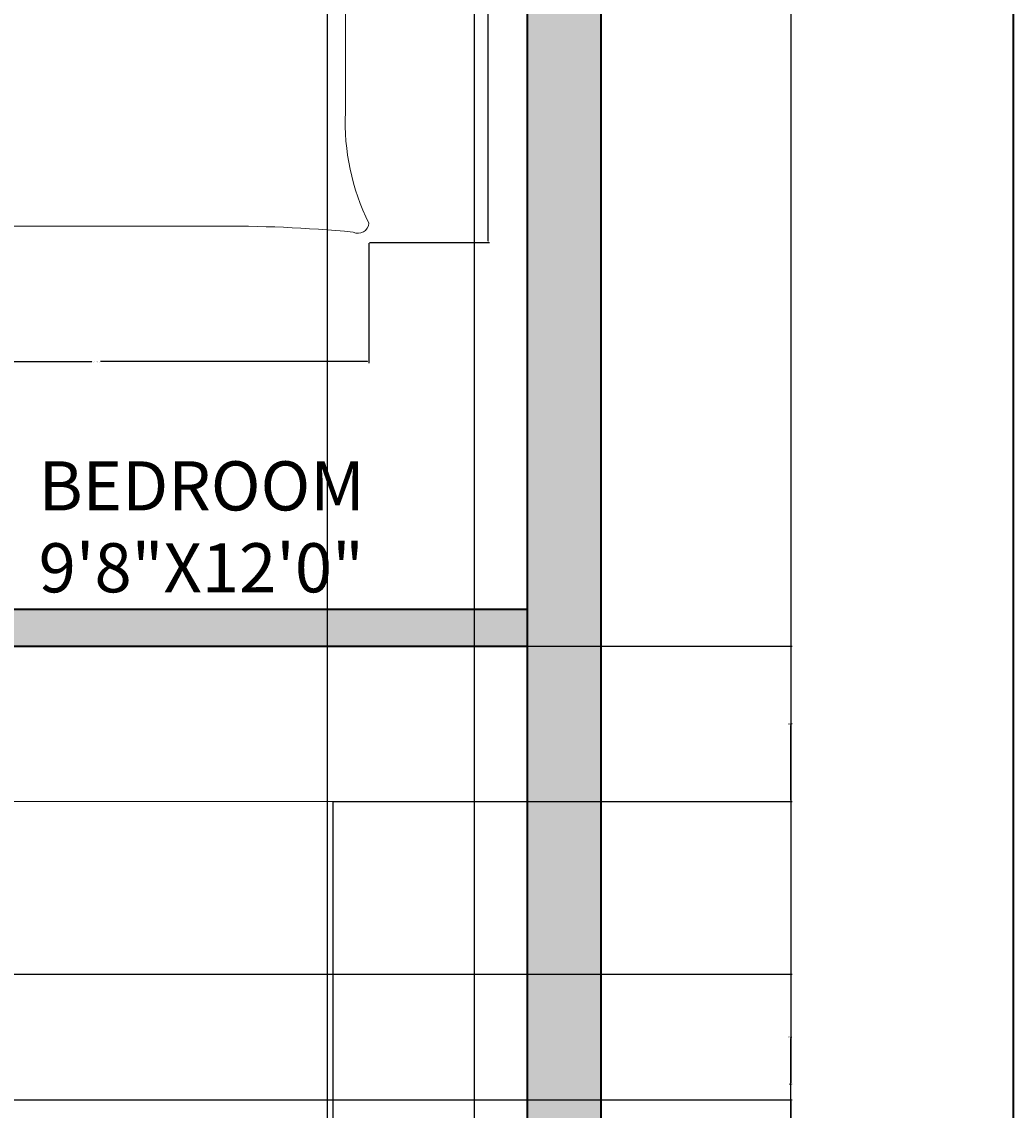
# Model space of a CAD drawing. Units: inches. Extents: x 2606 to 3027, y 1906 to 2463.
# Tile 8 of 10: x 2906 to 3027, y 2196 to 2329. Entities that reach past the tile are written whole.
import ezdxf

# ---------------------------------------------------------------- set-up
doc = ezdxf.new("R2010")
doc.units = ezdxf.units.IN
for name, color, linetype, lineweight in [('A-ANNO-DIMS', 2, 'Continuous', 18), ('A-ANNO-TTLB', 7, 'Continuous', 35), ('A-AREA-IDEN', 7, 'Continuous', 18), ('A-FLOR-CASE', 8, 'Continuous', 18), ('A-FURN', 8, 'Continuous', 13), ('A-WALL', 7, 'Continuous', 35)]:
    doc.layers.add(name, color=color, linetype=linetype, lineweight=lineweight)
doc.layers.add('A-WALL-PATT', color=251, linetype='Continuous', lineweight=13, true_color=0x636466)
doc.styles.get("Standard").update_dxf_attribs({"font": 'arial.ttf'})
doc.dimstyles.get("Standard").update_dxf_attribs({"dimtxt": 0.18, "dimasz": 0.18, "dimexe": 0.18, "dimexo": 0.0625, "dimgap": 0.09, "dimtad": 0, "dimtih": 1, "dimtoh": 1, "dimdec": 4, "dimzin": 0, "dimdsep": 46, "dimtxsty": 'Standard', "dimcen": 0.09, "dimadec": 0, "dimazin": 0, "dimtfac": 1, "dimtdec": 4, "dimtofl": 0, "dimtmove": 0, "dimatfit": 3, "dimfxl": 1, "dimtolj": 1, "dimtzin": 0, "dimarcsym": 0})

# ---------------------------------------------------------------- blocks, each defined once
blk = doc.blocks.new('BED-DOUBLE')
for p, q in [((4.17, 75.16), (4.17, 96.87)), ((4.17, 96.87), (61.46, 96.87)), ((61.46, 96.87), (61.46, 64.97)), ((4.17, 95.03), (61.46, 95.03)), ((29.42, 93.94), (31.15, 94.63)), ((31.15, 94.63), (31.84, 88.22)), ((4.67, 92.87), (9.81, 93.27)), ((9.81, 93.27), (9.93, 93.24)), ((9.93, 93.24), (14.52, 92.9)), ((17.81, 92.38), (20.24, 93.24)), ((20.24, 93.24), (23.7, 94.11)), ((23.7, 94.11), (24.09, 94.11)), ((24.09, 94.11), (29.42, 93.94)), ((33.54, 93.89), (33.25, 87.44)), ((35.31, 93.3), (33.54, 93.89)), ((40.62, 93.81), (35.31, 93.3)), ((41.01, 93.83), (40.62, 93.81)), ((44.52, 93.18), (41.01, 93.83)), ((50.25, 93.19), (43.75, 91.57)), ((47, 92.47), (44.52, 93.18)), ((54.8, 93.82), (50.25, 93.19)), ((60.08, 93.81), (53.6, 93.92)), ((53.6, 93.92), (54.8, 93.82)), ((60.08, 93.81), (59.62, 89.96)), ((4.67, 92.9), (5.36, 89.08)), ((14.52, 92.9), (21.1, 91.68)), ((5.36, 89.08), (4.84, 85.96)), ((6.06, 86.14), (7.27, 89.43)), ((59.12, 86.97), (57.7, 90.18)), ((59.62, 89.96), (60.34, 86.88)), ((31.84, 88.22), (32.54, 84.4)), ((33.25, 87.44), (32.79, 83.59)), ((60.08, 82.69), (59.12, 86.97)), ((60.34, 86.88), (59.72, 85.62)), ((4.84, 85.96), (5.54, 84.75)), ((5.36, 81.8), (6.06, 86.14)), ((32.54, 84.4), (32.54, 82.84)), ((32.54, 82.84), (31.84, 80.59)), ((32.79, 83.59), (32.89, 82.03)), ((59.85, 80.77), (60.08, 82.69)), ((5.71, 79.9), (5.36, 81.8)), ((32.89, 82.03), (33.72, 79.83)), ((5.02, 76.08), (5.71, 79.9)), ((31.84, 80.59), (31.84, 77.38)), ((33.72, 79.83), (33.92, 76.62)), ((60.78, 77), (59.85, 80.77)), ((28.9, 77.38), (25.13, 78.68)), ((7.65, 78.14), (12.48, 77.34)), ((12.48, 77.34), (11.13, 76.95)), ((12.48, 77.34), (20.89, 76.82)), ((20.89, 76.82), (23.24, 77.49)), ((23.24, 77.49), (29.39, 77)), ((31.84, 77.38), (28.9, 77.38)), ((36.87, 76.8), (40.55, 78.34)), ((39.04, 78.14), (43.87, 77.34)), ((43.87, 77.34), (52.28, 76.82)), ((52.28, 76.82), (54.63, 77.49)), ((54.63, 77.49), (60.78, 77)), ((11.13, 76.95), (5.02, 76.08)), ((33.92, 76.62), (36.87, 76.8)), ((36.28, 76.03), (41.3, 68.25)), ((48.73, 72.52), (38.73, 76.03)), ((55.41, 70.1), (48.73, 72.52)), ((58.94, 67.51), (55.41, 70.1)), ((41.3, 68.25), (43.34, 62.87)), ((63.38, 63.61), (58.94, 67.51)), ((43.34, 62.87), (43.71, 60.45)), ((49.1, 62.31), (53.18, 62.87)), ((53.18, 62.87), (57.82, 63.24)), ((57.82, 63.24), (61.54, 62.87)), ((61.54, 62.87), (63.38, 63.61)), ((63.48, 61.52), (63.38, 63.61, 4.64)), ((43.71, 60.45), (46.68, 61.2)), ((46.68, 61.2), (49.1, 62.31)), ((18.06, 1.87), (47.57, 1.87))]:
    blk.add_line(p, q)
for centre, radius, start, end in [((25.61, -121.38), 197.77, 86.0865, 96.7821), ((102.1, 72.78), 99.87, 178.7218, 185.604), ((21.29, -90.53), 154.68, 81.7845, 96.9006), ((-200.58, 59.5), 203.94, 358.4762, 1.0082), ((37.35, 95.1), 35.55, 280.6617, 289.8806), ((52.44, 54.83), 7.46, 78.6608, 113.7384), ((61.53, 104.85), 43.38, 259.8763, 272.5657), ((218.51, 53.34), 155.25, 176.9791, 183.8365), ((43.92, 60.38), 0.221, 160.2464, 271.1377), ((581.23, 36.19), 578.22, 178.22771, 181.71854), ((-5405.34, 15.56), 5469.02, 0.00217, 0.28689), ((-32.25, 19.53), 35.53, 346.0648, 358.9113), ((91.3, 14.55), 27.65, 177.4714, 206.4681), ((-25.97, 12.62), 28.25, 337.9751, 356.652), ((-20.65, 125.3), 127.63, 283.3832, 287.7053), ((1.3, 1.3), 1.31, 146.1736, 293.4781), ((25.69, -143.9), 145.97, 92.9958, 99.4091), ((49.34, -157.62), 159.5, 84.4998, 90.6351), ((65.23, 2.32), 1.32, 242.6588, 356.02)]:
    blk.add_arc(centre, radius, start, end)
blk = doc.blocks.new('*D9')
at = {"layer": 'A-ANNO-DIMS', "color": 0, "lineweight": -2, "transparency": 16777216}
for p, q in [((2948.82, 2399.4), (2963.48, 2399.4)), ((2963.3, 2399.22), (2963.3, 2351.08)), ((2963.3, 2302.58), (2963.3, 2350.71)), ((2948.82, 2302.4), (2963.48, 2302.4))]:
    blk.add_line(p, q, dxfattribs=at)
at = {"layer": 'A-ANNO-DIMS', "color": 0, "transparency": 16777216}
for points in [[(2963.27, 2399.22), (2963.33, 2399.22), (2963.3, 2399.4)], [(2963.27, 2302.58), (2963.33, 2302.58), (2963.3, 2302.4)]]:
    blk.add_solid(points, dxfattribs=at)
at = {"layer": 'Defpoints', "color": 0, "transparency": 16777216}
for p in [(2948.75, 2399.4), (2963.3, 2399.4), (2948.75, 2302.4)]:
    blk.add_point(p, dxfattribs=at)
at = {"layer": 'A-ANNO-DIMS', "color": 0, "transparency": 16777216, "insert": (2963.3, 2350.9), "char_height": 0.18, "attachment_point": 5}
blk.add_mtext('\\A1;DOUBLE BED 97 TYP.', dxfattribs=at)
blk = doc.blocks.new('*D10')
at = {"layer": 'A-ANNO-DIMS', "color": 0, "lineweight": -2, "transparency": 16777216}
for p, q in [((2882.1, 2302.34), (2882.1, 2287.67)), ((2948.75, 2302.34), (2948.75, 2287.67)), ((2882.28, 2287.85), (2914.9, 2287.85)), ((2948.57, 2287.85), (2915.96, 2287.85))]:
    blk.add_line(p, q, dxfattribs=at)
at = {"layer": 'A-ANNO-DIMS', "color": 0, "transparency": 16777216}
for points in [[(2882.28, 2287.88), (2882.28, 2287.82), (2882.1, 2287.85)], [(2948.57, 2287.88), (2948.57, 2287.82), (2948.75, 2287.85)]]:
    blk.add_solid(points, dxfattribs=at)
at = {"layer": 'Defpoints', "color": 0, "transparency": 16777216}
for p in [(2882.1, 2302.4), (2948.75, 2302.4), (2948.75, 2287.85)]:
    blk.add_point(p, dxfattribs=at)
at = {"layer": 'A-ANNO-DIMS', "color": 0, "transparency": 16777216, "insert": (2915.43, 2287.85), "char_height": 0.18, "attachment_point": 5}
blk.add_mtext('\\A1;67 TYP.', dxfattribs=at)
blk = doc.blocks.new('*D26')
at = {"layer": 'A-ANNO-DIMS', "color": 0, "lineweight": -2, "transparency": 16777216}
for p, q in [((2977.13, 2410.61), (3000.44, 2410.61)), ((3000.26, 2410.43), (3000.26, 2199.79)), ((3000.26, 1988.79), (3000.26, 2199.43)), ((2977.13, 1988.61), (3000.44, 1988.61))]:
    blk.add_line(p, q, dxfattribs=at)
at = {"layer": 'A-ANNO-DIMS', "color": 0, "transparency": 16777216}
for points in [[(3000.23, 2410.43), (3000.29, 2410.43), (3000.26, 2410.61)], [(3000.23, 1988.79), (3000.29, 1988.79), (3000.26, 1988.61)]]:
    blk.add_solid(points, dxfattribs=at)
at = {"layer": 'Defpoints', "color": 0, "transparency": 16777216}
for p in [(2977.06, 2410.61), (3000.26, 2410.61), (2977.06, 1988.61)]:
    blk.add_point(p, dxfattribs=at)
at = {"layer": 'A-ANNO-DIMS', "color": 0, "transparency": 16777216, "insert": (3000.26, 2199.61), "char_height": 0.18, "attachment_point": 5}
blk.add_mtext('\\A1;422', dxfattribs=at)
blk = doc.blocks.new('*D59')
at = {"layer": 'A-ANNO-DIMS', "color": 0, "lineweight": -2, "transparency": 16777216}
for p, q in [((2726.47, 2213.03), (3000.44, 2213.03)), ((3000.26, 2212.85), (3000.26, 2205.56)), ((3000.26, 2197.9), (3000.26, 2205.2)), ((2726.47, 2197.72), (3000.44, 2197.72))]:
    blk.add_line(p, q, dxfattribs=at)
at = {"layer": 'A-ANNO-DIMS', "color": 0, "transparency": 16777216}
for points in [[(3000.23, 2212.85), (3000.29, 2212.85), (3000.26, 2213.03)], [(3000.23, 2197.9), (3000.29, 2197.9), (3000.26, 2197.72)]]:
    blk.add_solid(points, dxfattribs=at)
at = {"layer": 'Defpoints', "color": 0, "transparency": 16777216}
for p in [(2726.4, 2213.03), (3000.26, 2213.03), (2726.4, 2197.72)]:
    blk.add_point(p, dxfattribs=at)
at = {"layer": 'A-ANNO-DIMS', "color": 0, "transparency": 16777216, "insert": (3000.26, 2205.38), "char_height": 0.18, "attachment_point": 5}
blk.add_mtext('\\A1;15.31', dxfattribs=at)
blk = doc.blocks.new('*D61')
at = {"layer": 'A-ANNO-DIMS', "color": 0, "lineweight": -2, "transparency": 16777216}
for p, q in [((2696.29, 2197.72), (3000.44, 2197.72)), ((3000.26, 2197.54), (3000.26, 2190.63)), ((3000.26, 2183.36), (3000.26, 2190.27)), ((2696.84, 2183.18), (3000.44, 2183.18))]:
    blk.add_line(p, q, dxfattribs=at)
at = {"layer": 'A-ANNO-DIMS', "color": 0, "transparency": 16777216}
for points in [[(3000.23, 2197.54), (3000.29, 2197.54), (3000.26, 2197.72)], [(3000.23, 2183.36), (3000.29, 2183.36), (3000.26, 2183.18)]]:
    blk.add_solid(points, dxfattribs=at)
at = {"layer": 'Defpoints', "color": 0, "transparency": 16777216}
for p in [(2696.23, 2197.72), (3000.26, 2197.72), (2696.78, 2183.18)]:
    blk.add_point(p, dxfattribs=at)
at = {"layer": 'A-ANNO-DIMS', "color": 0, "transparency": 16777216, "insert": (3000.26, 2190.45), "char_height": 0.18, "attachment_point": 5}
blk.add_mtext('\\A1;14.545', dxfattribs=at)
blk = doc.blocks.new('*D66')
at = {"layer": 'A-ANNO-DIMS', "color": 0, "lineweight": -2, "transparency": 16777216}
for p, q in [((2968.06, 2253.05), (2968.06, 1965.23)), ((2944.33, 2234.06), (2944.33, 1965.23)), ((2944.51, 1965.41), (2955.8, 1965.41)), ((2967.88, 1965.41), (2956.59, 1965.41))]:
    blk.add_line(p, q, dxfattribs=at)
at = {"layer": 'A-ANNO-DIMS', "color": 0, "transparency": 16777216}
for points in [[(2944.51, 1965.44), (2944.51, 1965.38), (2944.33, 1965.41)], [(2967.88, 1965.44), (2967.88, 1965.38), (2968.06, 1965.41)]]:
    blk.add_solid(points, dxfattribs=at)
at = {"layer": 'Defpoints', "color": 0, "transparency": 16777216}
for p in [(2968.06, 2253.11), (2944.33, 2234.12), (2968.06, 1965.41)]:
    blk.add_point(p, dxfattribs=at)
at = {"layer": 'A-ANNO-DIMS', "color": 0, "transparency": 16777216, "insert": (2956.2, 1965.41), "char_height": 0.18, "attachment_point": 5}
blk.add_mtext('\\A1;23.73', dxfattribs=at)
blk = doc.blocks.new('*D67')
at = {"layer": 'A-ANNO-DIMS', "color": 0, "lineweight": -2, "transparency": 16777216}
for p, q in [((2968.13, 2253.11), (3000.44, 2253.11)), ((3000.26, 2252.93), (3000.26, 2243.8)), ((3000.26, 2234.3), (3000.26, 2243.43)), ((2944.4, 2234.12), (3000.44, 2234.12))]:
    blk.add_line(p, q, dxfattribs=at)
at = {"layer": 'A-ANNO-DIMS', "color": 0, "transparency": 16777216}
for points in [[(3000.23, 2252.93), (3000.29, 2252.93), (3000.26, 2253.11)], [(3000.23, 2234.3), (3000.29, 2234.3), (3000.26, 2234.12)]]:
    blk.add_solid(points, dxfattribs=at)
at = {"layer": 'Defpoints', "color": 0, "transparency": 16777216}
for p in [(2968.06, 2253.11), (3000.26, 2253.11), (2944.33, 2234.12)]:
    blk.add_point(p, dxfattribs=at)
at = {"layer": 'A-ANNO-DIMS', "color": 0, "transparency": 16777216, "insert": (3000.26, 2243.62), "char_height": 0.18, "attachment_point": 5}
blk.add_mtext('\\A1;18.99', dxfattribs=at)
blk = doc.blocks.new('*D75')
at = {"layer": 'A-ANNO-DIMS', "color": 0, "lineweight": -2, "transparency": 16777216}
for p, q in [((2968.06, 2401.55), (2968.06, 1965.23)), ((2943.67, 2399.33), (2943.67, 1965.23)), ((2943.85, 1965.41), (2955.4, 1965.41)), ((2967.88, 1965.41), (2956.33, 1965.41))]:
    blk.add_line(p, q, dxfattribs=at)
at = {"layer": 'A-ANNO-DIMS', "color": 0, "transparency": 16777216}
for points in [[(2943.85, 1965.44), (2943.85, 1965.38), (2943.67, 1965.41)], [(2967.88, 1965.44), (2967.88, 1965.38), (2968.06, 1965.41)]]:
    blk.add_solid(points, dxfattribs=at)
at = {"layer": 'Defpoints', "color": 0, "transparency": 16777216}
for p in [(2968.06, 2401.61), (2943.67, 2399.4), (2968.06, 1965.41)]:
    blk.add_point(p, dxfattribs=at)
at = {"layer": 'A-ANNO-DIMS', "color": 0, "transparency": 16777216, "insert": (2955.86, 1965.41), "char_height": 0.18, "attachment_point": 5}
blk.add_mtext('\\A1;24.397', dxfattribs=at)
blk = doc.blocks.new('*D77')
at = {"layer": 'A-ANNO-DIMS', "color": 0, "lineweight": -2, "transparency": 16777216}
for p, q in [((2961.66, 2034.29), (2961.66, 2433.99)), ((2968.06, 2032.67), (2968.06, 2433.99)), ((2961.84, 2433.81), (2964.47, 2433.81)), ((2967.88, 2433.81), (2965.26, 2433.81))]:
    blk.add_line(p, q, dxfattribs=at)
at = {"layer": 'A-ANNO-DIMS', "color": 0, "transparency": 16777216}
for points in [[(2961.84, 2433.84), (2961.84, 2433.78), (2961.66, 2433.81)], [(2967.88, 2433.84), (2967.88, 2433.78), (2968.06, 2433.81)]]:
    blk.add_solid(points, dxfattribs=at)
at = {"layer": 'Defpoints', "color": 0, "transparency": 16777216}
for p in [(2968.06, 2433.81), (2961.66, 2034.23), (2968.06, 2032.61)]:
    blk.add_point(p, dxfattribs=at)
at = {"layer": 'A-ANNO-DIMS', "color": 0, "transparency": 16777216, "insert": (2964.86, 2433.81), "char_height": 0.18, "attachment_point": 5}
blk.add_mtext('\\A1;6.402', dxfattribs=at)

msp = doc.modelspace()

# ---------------------------------------------------------------- hatches: boundary and pattern name
at = {"layer": 'A-WALL-PATT'}
h = msp.add_hatch(color=256, dxfattribs=at)
h.dxf.hatch_style = 1
h.paths.add_polyline_path([(2667.063, 2401.6097), (2691.9697, 2401.6097), (2691.9697, 2406.1097), (2691.9697, 2410.6097), (2658.063, 2410.6097), (2658.063, 2238.7051), (2667.063, 2238.7051)])
h.paths.add_polyline_path([(2804.9965, 2406.1097), (2804.9965, 2410.6097), (2751.9697, 2410.6097), (2751.9697, 2401.6097), (2783.063, 2401.6097), (2783.063, 2257.6097), (2778.6739, 2257.6097), (2778.6739, 2253.1097), (2792.3386, 2253.1097), (2792.3386, 2255.3597), (2792.3386, 2257.6097), (2787.563, 2257.6097), (2787.563, 2327.1097), (2847.563, 2327.1097), (2847.563, 2331.6097), (2787.563, 2331.6097), (2787.563, 2401.6097), (2804.9965, 2401.6097)])
h.paths.add_polyline_path([(2889.6183, 2406.1097), (2889.6183, 2410.6097), (2828.9965, 2410.6097), (2828.9965, 2401.6097), (2831.8174, 2401.6097), (2847.563, 2401.6097), (2847.563, 2357.8311), (2849.813, 2357.8311), (2852.063, 2357.8311), (2852.063, 2401.6097), (2889.6183, 2401.6097)])
h.paths.add_polyline_path([(2977.063, 2410.6097), (2949.6183, 2410.6097), (2949.6183, 2401.6097), (2968.063, 2401.6097), (2968.063, 2157.1097), (2897.063, 2157.1097), (2897.063, 2174.1966), (2892.563, 2174.1966), (2892.563, 2157.1097), (2886.8122, 2157.1097), (2886.8122, 2152.6097), (2968.063, 2152.6097), (2968.063, 2032.6097), (2950.8911, 2032.6097), (2950.8911, 2028.1097), (2968.063, 2028.1097), (2968.063, 1993.1097), (2852.063, 1993.1097), (2852.063, 2028.1097), (2856.0743, 2028.1097), (2856.0743, 2030.3597), (2856.0743, 2032.6097), (2852.063, 2032.6097), (2852.063, 2152.6097), (2857.369, 2152.6097), (2857.369, 2154.8597), (2857.369, 2157.1097), (2847.563, 2157.1097), (2847.563, 2152.6097), (2847.563, 1993.1097), (2837.0415, 1993.1097), (2837.0415, 1988.6097), (2977.063, 1988.6097)])
h.paths.add_polyline_path([(2968.063, 2257.6097), (2886.9679, 2257.6097), (2886.9679, 2253.1097), (2892.563, 2253.1097), (2892.563, 2215.1332), (2897.063, 2215.1332), (2897.063, 2253.1097), (2968.063, 2253.1097)], flags=17)
h.paths.add_polyline_path([(2856.057, 2255.3597), (2856.057, 2257.6097), (2852.063, 2257.6097), (2852.063, 2336.7476), (2849.813, 2336.7476), (2847.563, 2336.7476), (2847.563, 2331.6097), (2847.563, 2327.1097), (2847.563, 2257.6097), (2813.482, 2257.6097), (2813.482, 2253.1097), (2856.057, 2253.1097)])
h.paths.add_polyline_path([(2748.8874, 2255.3597), (2748.8874, 2257.6097), (2667.063, 2257.6097), (2667.063, 2253.1097), (2748.8874, 2253.1097)])
h.paths.add_polyline_path([(2667.063, 2152.6097), (2744.8238, 2152.6097), (2744.8238, 2154.8597), (2744.8238, 2157.1097), (2667.063, 2157.1097), (2667.063, 2178.7051), (2658.063, 2178.7051), (2658.063, 1988.6097), (2801.0415, 1988.6097), (2801.0415, 1990.8597), (2801.0415, 1993.1097), (2787.563, 1993.1097), (2787.563, 2157.1097), (2777.1295, 2157.1097), (2777.1295, 2152.6097), (2783.063, 2152.6097), (2783.063, 2032.6097), (2778.4484, 2032.6097), (2778.4484, 2028.1097), (2783.063, 2028.1097), (2783.063, 1993.1097), (2667.063, 1993.1097), (2667.063, 2028.1097), (2680.1652, 2028.1097), (2680.1652, 2030.3597), (2680.1652, 2032.6097), (2667.063, 2032.6097)])
h.paths.add_polyline_path([(2755.4074, 2032.6097), (2728.1652, 2032.6097), (2728.1652, 2028.1097), (2755.4074, 2028.1097), (2755.4074, 2030.3597)], flags=17)
h.paths.add_polyline_path([(2902.8911, 2030.3597), (2902.8911, 2032.6097), (2877.6885, 2032.6097), (2877.6885, 2028.1097), (2902.8911, 2028.1097)], flags=17)
h.paths.add_polyline_path([(2810.2211, 2267.221), (2851.2716, 2267.221), (2851.2716, 2289.6098), (2810.2211, 2289.6098)], flags=9)

# ---------------------------------------------------------------- linework, layer by layer
at = {"layer": 'A-ANNO-TTLB'}
msp.add_lwpolyline([(2605.9227, 2462.7868), (3027.4339, 2462.7868), (3027.4339, 1905.5336), (2605.9227, 1905.5336)], close=True, dxfattribs=at)
at = {"layer": 'A-FLOR-CASE'}
for p, q in [((2897.063, 2234.1214), (2944.3333, 2234.1214)), ((2944.3333, 2234.1214), (2944.3333, 2157.1097))]:
    msp.add_line(p, q, dxfattribs=at)
at = {"layer": 'A-WALL'}
for p, q in [((2977.063, 2410.6097), (2977.063, 1988.6097)), ((2968.063, 2401.6097), (2968.063, 2157.1097)), ((2885.5319, 2257.6097), (2968.063, 2257.6097)), ((2897.063, 2253.1097), (2968.063, 2253.1097))]:
    msp.add_line(p, q, dxfattribs=at)

# ---------------------------------------------------------------- block references
at = {"layer": 'A-FURN'}
msp.add_blockref('BED-DOUBLE', (2882.206, 2302.524), dxfattribs=at)

# ---------------------------------------------------------------- texts
at = {"layer": 'A-AREA-IDEN', "insert": (2908.4167, 2275.68), "char_height": 6, "attachment_point": 1}
msp.add_mtext_dynamic_manual_height_columns('BEDROOM\\P9\'8"X12\'0"', width=79.441343, gutter_width=12.5, heights=[0], dxfattribs=at)

# ---------------------------------------------------------------- dimensions: what is measured, and where the dimension line sits
at = {"layer": 'A-ANNO-DIMS'}
for base, p1, p2, override, picture, middle in [((2968.063, 2433.8097), (2961.6611, 2034.2301), (2968.063, 2032.6097), {"dimdec": 3, "dimlfac": 1, "dimrnd": 0, "dimzin": 0, "dimdsep": 46, "dimlunit": 2}, '*D77', (2964.8621, 2433.8097)), ((2968.063, 1965.4097), (2943.6661, 2399.3963), (2968.063, 2401.6097), {"dimdec": 3, "dimlfac": 1, "dimrnd": 0, "dimzin": 0, "dimdsep": 46, "dimlunit": 2}, '*D75', (2955.8645, 1965.4097)), ((2968.063, 1965.4097), (2944.3333, 2234.1214), (2968.063, 2253.1097), {"dimdec": 2, "dimlfac": 1, "dimrnd": 0, "dimzin": 0, "dimdsep": 46, "dimlunit": 2}, '*D66', (2956.1982, 1965.4097))]:
    dim = msp.add_linear_dim(base=base, p1=p1, p2=p2, dimstyle='Standard', override=override, dxfattribs=at)
    dim.commit()
    dim.dimension.update_dxf_attribs({"geometry": picture, "text_midpoint": middle})
for base, p1, p2, override, picture, middle in [((3000.263, 2410.6097), (2977.063, 1988.6097), (2977.063, 2410.6097), {"dimdec": 0, "dimlfac": 1, "dimrnd": 0, "dimzin": 0, "dimdsep": 46, "dimlunit": 2}, '*D26', (3000.263, 2199.6097)), ((3000.263, 2253.1097), (2944.3333, 2234.1214), (2968.063, 2253.1097), {"dimdec": 2, "dimlfac": 1, "dimrnd": 0, "dimzin": 0, "dimdsep": 46, "dimlunit": 2}, '*D67', (3000.263, 2243.6156)), ((3000.263, 2213.0343), (2726.4032, 2197.7249), (2726.4032, 2213.0343), {"dimdec": 2, "dimlfac": 1, "dimrnd": 0, "dimzin": 0, "dimdsep": 46, "dimlunit": 2}, '*D59', (3000.263, 2205.3796)), ((3000.263, 2197.7249), (2696.782, 2183.1802), (2696.232, 2197.7249), {"dimdec": 3, "dimlfac": 1, "dimrnd": 0, "dimzin": 0, "dimdsep": 46, "dimlunit": 2}, '*D61', (3000.263, 2190.4526))]:
    dim = msp.add_linear_dim(base=base, p1=p1, p2=p2, angle=90, dimstyle='Standard', override=override, dxfattribs=at)
    dim.commit()
    dim.dimension.update_dxf_attribs({"geometry": picture, "text_midpoint": middle})
dim = msp.add_linear_dim(base=(2963.3041, 2399.3963), p1=(2948.7543, 2302.3976), p2=(2948.7543, 2399.3963), angle=90, text='DOUBLE BED <> TYP.', dimstyle='Standard', override={"dimdec": 0, "dimlfac": 1, "dimrnd": 0, "dimzin": 0, "dimdsep": 46, "dimlunit": 2}, dxfattribs=at)
dim.commit()
dim.dimension.update_dxf_attribs({"geometry": '*D9', "text_midpoint": (2963.3041, 2350.897)})
dim = msp.add_linear_dim(base=(2948.7543, 2287.8478), p1=(2882.1028, 2302.3976), p2=(2948.7543, 2302.3976), text='<> TYP.', dimstyle='Standard', override={"dimdec": 0, "dimlfac": 1, "dimrnd": 0, "dimzin": 0, "dimdsep": 46, "dimlunit": 2}, dxfattribs=at)
dim.commit()
dim.dimension.update_dxf_attribs({"geometry": '*D10', "text_midpoint": (2915.4285, 2287.8478)})

doc.saveas('drawing.dxf')
